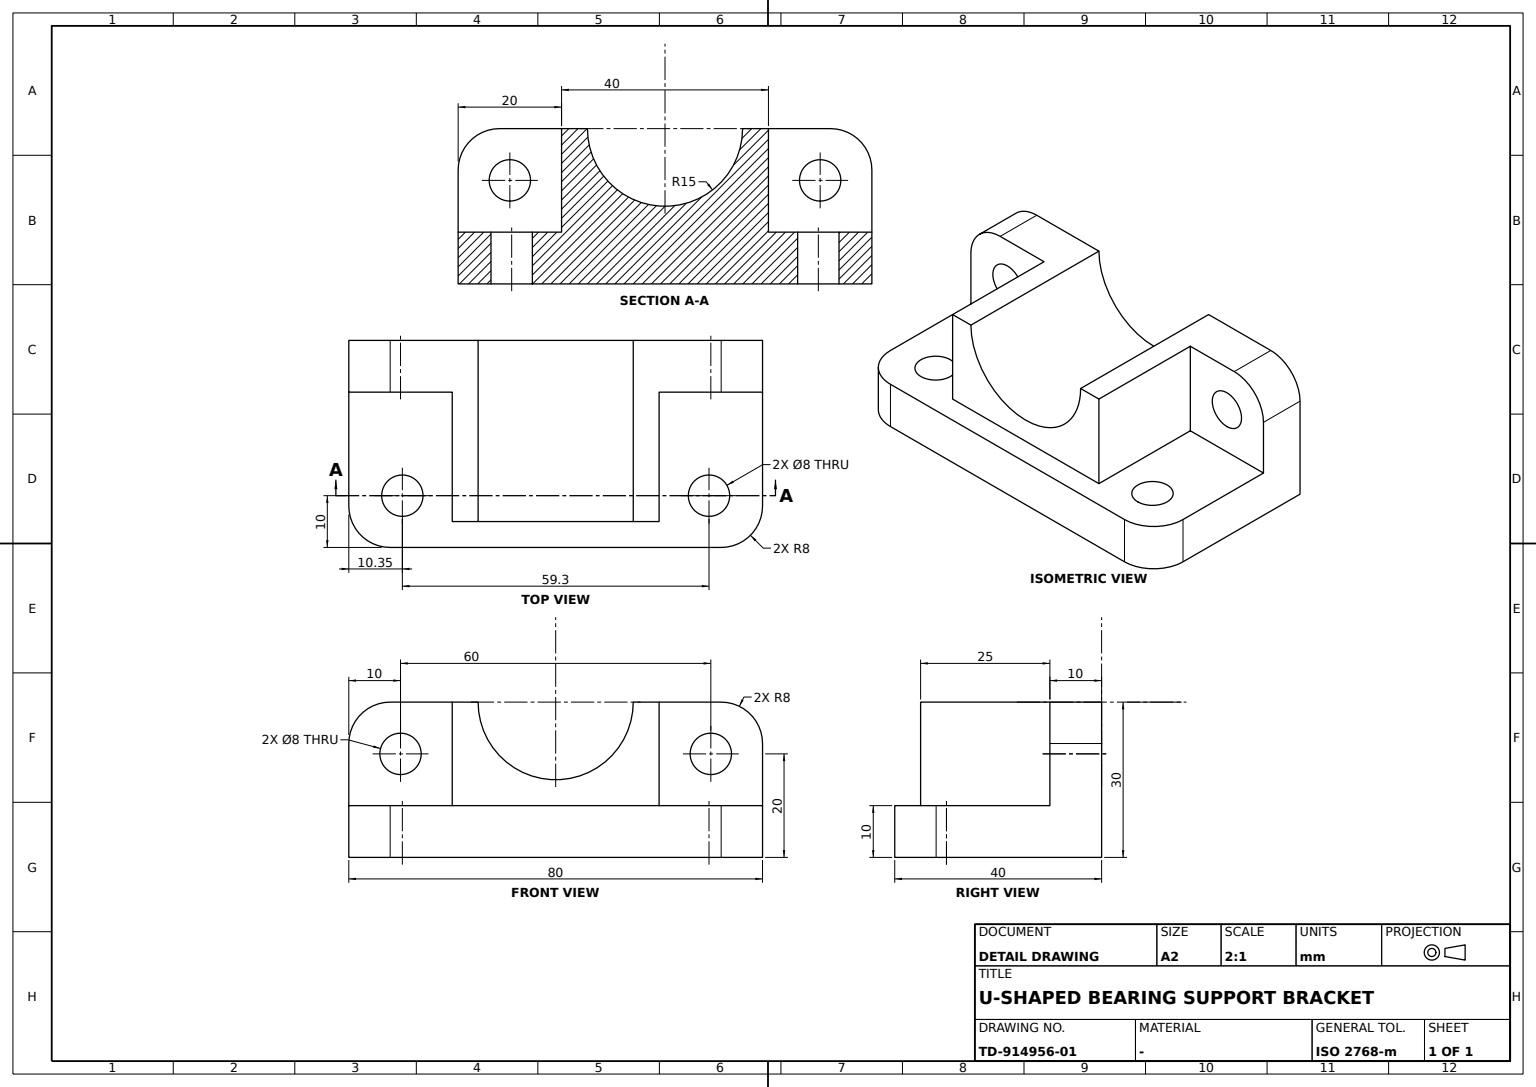
CATIA V5 part; units mm, degrees
sketch "Sketch1" plane through (0, 0, 0) normal (1, 0, 0) x (0, 1, 0)
  line L0 (40, 15) -> (40, -15)
  line L1 (40, -15) -> (-40, -15)
  line L2 (-40, -15) -> (-40, 15)
  line L3 (-40, 15) -> (40, 15)
  circle A0 centre (-30, 5) radius 4
  point P0 (-30, 9)
  circle A1 centre (30, 5) radius 4
  dimension "distance L1 L3" = 30
  dimension "distance L0 L2" = 80
  dimension "distance P0 y axis" = 30
  dimension "radius A0" = 4
  constraint vertical L0 y-axis
  constraint vertical L2 y-axis
  constraint horizontal L1 x-axis
  constraint horizontal L3 x-axis
  constraint equidistance L0 L2 origin
  constraint equidistance L1 L3 origin
  constraint coincidence A0 P0
  constraint symmetry A0 A1 y-axis
extrude "Pad1" add sketch "Sketch1" along normal blind 10
fillet "Fillet1" radius 8 1 edges at (5, 40, 15)
fillet "Fillet2" radius 8 1 edges at (5, -40, 15)
sketch "Sketch2" plane through (10, 0, 0) normal (1, 0, 0) x (0, 1, 0)
  line L0 (40, -15) -> (40, -5)
  line L1 (40, -5) -> (-40, -5)
  line L2 (-40, -5) -> (-40, -15)
  line L3 (-40, -15) -> (40, -15)
  dimension "length L1" = 80
  dimension "length L2" = 10
  constraint vertical L0 y-axis
  constraint vertical L2 y-axis
  constraint horizontal L1 x-axis
  constraint horizontal L3 x-axis
extrude "Pad2" add sketch "Sketch2" along normal blind 30
fillet "Fillet3" radius 8 1 edges at (40, 40, -10)
fillet "Fillet4" radius 8 1 edges at (40, -40, -10)
sketch "Sketch3" plane through (0, 0, -5) normal (0, 0, 1) x (1, 0, 0)
  circle A0 centre (30, 29.6481) radius 4
  circle A1 centre (30, -29.6481) radius 4
  dimension "radius A0" = 4
extrude "Pocket1" cut sketch "Sketch3" against normal through all
sketch "Sketch4" plane through (10, 0, 0) normal (1, 0, 0) x (0, 1, 0)
  line L0 (-20, 15) -> (20, 15)
  line L1 (-20, 15) -> (-20, -5)
  line L2 (20, 15) -> (20, -5)
  line L3 (20, -5) -> (-20, -5)
  dimension "length L1" = 20
  constraint horizontal L0 x-axis
  constraint horizontal L3 x-axis
  constraint vertical L1 y-axis
  constraint vertical L2 y-axis
extrude "Pad3" add sketch "Sketch4" along normal blind 25
sketch "Sketch5" plane through (35, 0, 0) normal (1, 0, 0) x (0, 1, 0)
  circle A0 centre (0, 15) radius 15
  point P0 (0, 0)
  constraint coincidence A0 P0
  constraint coincidence P0 x-axis
  constraint coincidence A0 origin
extrude "Pocket2" cut sketch "Sketch5" against normal through all
